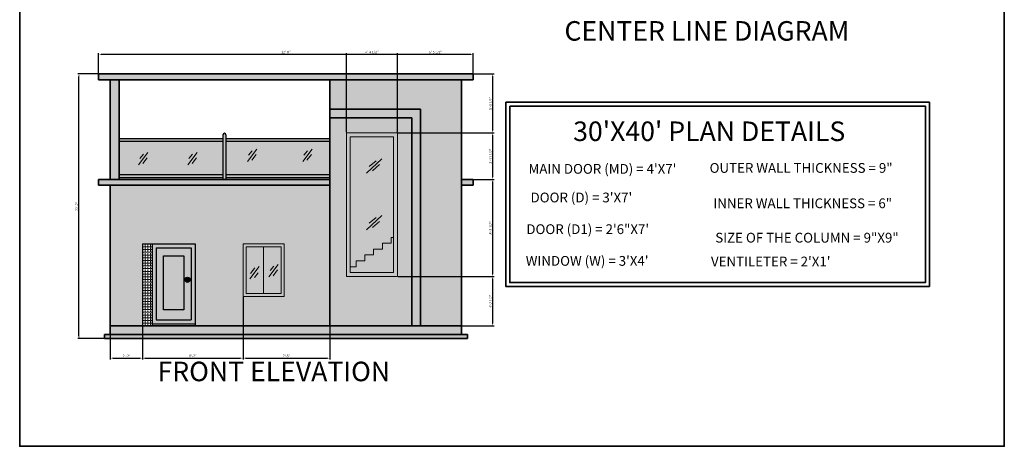
# Model space of a CAD drawing. Units: inches. Extents: x 2150 to 10686, y 1035 to 5077.
# Tile 1 of 12: x 2150 to 3159, y 1035 to 1472. Entities that reach past the tile are written whole.
import ezdxf

# ---------------------------------------------------------------- set-up
doc = ezdxf.new("R2010")
doc.units = ezdxf.units.IN
for name, color, linetype, lineweight in [('A-ANNO-DIMS', 2, 'Continuous', 18), ('A-ANNO-TEXT', 2, 'Continuous', 18), ('A-ANNO-TITL', 3, 'Continuous', 35), ('A-ANNO-TTLB', 7, 'Continuous', 35), ('A-ELEV', 7, 'Continuous', 35), ('A-ELEV-BASE-PATT', 251, 'Continuous', 13), ('A-ELEV-DOOR', 7, 'Continuous', 25), ('A-ELEV-DOOR-PATT', 17, 'Continuous', 13), ('A-ELEV-GLAZ', 7, 'Continuous', 18), ('A-ELEV-MASN-PATT', 32, 'Continuous', 13), ('A-ELEV-METL-PATT', 252, 'Continuous', 13), ('A-ELEV-RAIL', 7, 'Continuous', 25), ('A-ELEV-STRS', 7, 'Continuous', 18)]:
    doc.layers.add(name, color=color, linetype=linetype, lineweight=lineweight)
for name, color, linetype, lineweight, true_color in [('A-ELEV-CONC-PATT', 253, 'Continuous', 13, 0xb2a88f), ('A-ELEV-GLAZ-PATT', 141, 'Continuous', 13, 0xadddf7), ('A-ELEV-PATT', 253, 'Continuous', 13, 0xa5adc8)]:
    doc.layers.add(name, color=color, linetype=linetype, lineweight=lineweight, true_color=true_color)
doc.styles.get("Standard").update_dxf_attribs({"font": 'arial.ttf'})
doc.dimstyles.new('ISO-25', dxfattribs={"dimtxt": 2.5, "dimasz": 2.5, "dimexe": 1.25, "dimexo": 0.625, "dimtad": 1, "dimdec": 0, "dimlunit": 3, "dimtxsty": 'Standard', "dimcen": 2.5, "dimadec": 0, "dimazin": 0, "dimtfac": 1, "dimtdec": 0, "dimtmove": 0, "dimatfit": 3, "dimfxl": 1, "dimarcsym": 0})
pattern_1 = [(50, (-2138.8083, -54.4876), (3.6436934, -0.3187817), [0.381, -4.191]), (355, (-2138.8083, -54.4876), (-0.7048684, 3.821137), [0.3048, -3.3528117]), (100.451445, (-2138.5047, -54.514), (2.938825, 3.502355), [0.3238002, -3.561805]), (46.1842, (-2138.8083, -53.4716), (5.421581, -0.8408466), [0.5715, -6.2865]), (96.63556, (-2138.3565, -53.5416), (4.7480827, 4.9485225), [0.4857005, -5.342712]), (351.18415, (-2138.8083, -53.4716), (4.7480827, 4.9485225), [0.4571993, -5.0291946]), (21, (-2138.3003, -53.7256), (3.0322878, -2.045304), [0.381, -4.191]), (326, (-2138.3003, -53.7256), (1.2360406, 3.6837593), [0.3048, -3.3528]), (71.451445, (-2138.0476, -53.896), (4.2683284, 1.6384554), [0.3238002, -3.5617988]), (37.5, (-2138.8083, -54.4876), (0.06177207, 1.69110078), [0, -3.31216, 0, -3.4036, 0, -3.3655]), (7.5, (-2138.8083, -54.4876), (1.33639325, 2.0036115), [0, -1.94056, 0, -3.23596, 0, -1.2827]), (327.5, (-2139.9412, -54.4876), (2.7118119, -0.11457488), [0, -1.27, 0, -3.9624, 0, -5.2578]), (317.5, (-2140.4492, -54.4876), (2.9625836, 0.5085298), [0, -1.651, 0, -2.63144, 0, -3.7338])]

# ---------------------------------------------------------------- blocks, each defined once
blk = doc.blocks.new('GLASS-REFLECTION-SLIM')
for p, q in [((0, 0), (9.4, 12.8)), ((0.6, 5.5), (5.1, 11.4)), ((4.6, 1.7), (8.3, 6.2))]:
    blk.add_line(p, q)
blk = doc.blocks.new('GLASS-REFLECTION-TALL')
for p, q in [((0, 0), (15.7, 14.7)), ((2.4, 6.8), (9.9, 12.7)), ((6.1, 2.4), (13.3, 8.7))]:
    blk.add_line(p, q)
blk = doc.blocks.new('*D103')
at = {"layer": 'A-ANNO-DIMS', "color": 0, "lineweight": -2, "transparency": 16777216}
for p, q in [((2230.7, 1416.8), (2230.7, 1437.5)), ((2233.2, 1436.3), (2612.2, 1436.3)), ((2614.7, 1416.8), (2614.7, 1437.5))]:
    blk.add_line(p, q, dxfattribs=at)
at = {"layer": 'A-ANNO-DIMS', "color": 0, "transparency": 16777216}
for points in [[(2233.2, 1436.7), (2233.2, 1435.9), (2230.7, 1436.3)], [(2612.2, 1436.7), (2612.2, 1435.9), (2614.7, 1436.3)]]:
    blk.add_solid(points, dxfattribs=at)
at = {"layer": 'Defpoints', "color": 0, "transparency": 16777216}
for p in [(2614.7, 1436.3), (2230.7, 1416.2), (2614.7, 1416.2)]:
    blk.add_point(p, dxfattribs=at)
at = {"layer": 'A-ANNO-DIMS', "color": 0, "transparency": 16777216, "insert": (2422.7, 1438.2), "char_height": 2.5, "attachment_point": 5}
blk.add_mtext('32\'-0"', dxfattribs=at)
blk = doc.blocks.new('*D104')
at = {"layer": 'A-ANNO-DIMS', "color": 0, "lineweight": -2, "transparency": 16777216}
for p, q in [((2230.1, 1416.2), (2209.4, 1416.2)), ((2210.6, 1147.7), (2210.6, 1413.7)), ((2236.1, 1145.2), (2209.4, 1145.2))]:
    blk.add_line(p, q, dxfattribs=at)
at = {"layer": 'A-ANNO-DIMS', "color": 0, "transparency": 16777216}
for points in [[(2210.2, 1413.7), (2211.1, 1413.7), (2210.6, 1416.2)], [(2210.2, 1147.7), (2211.1, 1147.7), (2210.6, 1145.2)]]:
    blk.add_solid(points, dxfattribs=at)
at = {"layer": 'Defpoints', "color": 0, "transparency": 16777216}
for p in [(2210.6, 1416.2), (2230.7, 1416.2), (2236.7, 1145.2)]:
    blk.add_point(p, dxfattribs=at)
at = {"layer": 'A-ANNO-DIMS', "color": 0, "transparency": 16777216, "insert": (2208.8, 1280.7), "char_height": 2.5, "attachment_point": 5, "rotation": 90}
blk.add_mtext('22\'-7"', dxfattribs=at)
blk = doc.blocks.new('*D105')
at = {"layer": 'A-ANNO-DIMS', "color": 0, "lineweight": -2, "transparency": 16777216}
for p, q in [((2537.6, 1208.8), (2636, 1208.8)), ((2634.7, 1160.7), (2634.7, 1206.3)), ((2603.3, 1158.2), (2636, 1158.2))]:
    blk.add_line(p, q, dxfattribs=at)
at = {"layer": 'A-ANNO-DIMS', "color": 0, "transparency": 16777216}
for points in [[(2634.3, 1206.3), (2635.2, 1206.3), (2634.7, 1208.8)], [(2634.3, 1160.7), (2635.2, 1160.7), (2634.7, 1158.2)]]:
    blk.add_solid(points, dxfattribs=at)
at = {"layer": 'Defpoints', "color": 0, "transparency": 16777216}
for p in [(2537, 1208.8), (2634.7, 1208.8), (2602.7, 1158.2)]:
    blk.add_point(p, dxfattribs=at)
at = {"layer": 'A-ANNO-DIMS', "color": 0, "transparency": 16777216, "insert": (2632.8, 1183.5), "char_height": 2.5, "attachment_point": 5, "rotation": 90}
blk.add_mtext('4\'-2 1/2"', dxfattribs=at)
blk = doc.blocks.new('*D106')
at = {"layer": 'A-ANNO-DIMS', "color": 0, "lineweight": -2, "transparency": 16777216}
for p, q in [((2615.3, 1308.2), (2636, 1308.2)), ((2634.7, 1211.3), (2634.7, 1305.7)), ((2537.6, 1208.8), (2636, 1208.8))]:
    blk.add_line(p, q, dxfattribs=at)
at = {"layer": 'A-ANNO-DIMS', "color": 0, "transparency": 16777216}
for points in [[(2634.3, 1305.7), (2635.2, 1305.7), (2634.7, 1308.2)], [(2634.3, 1211.3), (2635.2, 1211.3), (2634.7, 1208.8)]]:
    blk.add_solid(points, dxfattribs=at)
at = {"layer": 'Defpoints', "color": 0, "transparency": 16777216}
for p in [(2614.7, 1308.2), (2634.7, 1308.2), (2537, 1208.8)]:
    blk.add_point(p, dxfattribs=at)
at = {"layer": 'A-ANNO-DIMS', "color": 0, "transparency": 16777216, "insert": (2632.8, 1258.5), "char_height": 2.5, "attachment_point": 5, "rotation": 90}
blk.add_mtext('8\'-3 1/2"', dxfattribs=at)
blk = doc.blocks.new('*D107')
at = {"layer": 'A-ANNO-DIMS', "color": 0, "lineweight": -2, "transparency": 16777216}
for p, q in [((2537.6, 1355.9), (2636, 1355.9)), ((2634.7, 1310.7), (2634.7, 1353.4)), ((2615.3, 1308.2), (2636, 1308.2))]:
    blk.add_line(p, q, dxfattribs=at)
at = {"layer": 'A-ANNO-DIMS', "color": 0, "transparency": 16777216}
for points in [[(2634.3, 1353.4), (2635.2, 1353.4), (2634.7, 1355.9)], [(2634.3, 1310.7), (2635.2, 1310.7), (2634.7, 1308.2)]]:
    blk.add_solid(points, dxfattribs=at)
at = {"layer": 'Defpoints', "color": 0, "transparency": 16777216}
for p in [(2537, 1355.9), (2634.7, 1355.9), (2614.7, 1308.2)]:
    blk.add_point(p, dxfattribs=at)
at = {"layer": 'A-ANNO-DIMS', "color": 0, "transparency": 16777216, "insert": (2632.8, 1332), "char_height": 2.5, "attachment_point": 5, "rotation": 90}
blk.add_mtext('3\'-11 1/2"', dxfattribs=at)
blk = doc.blocks.new('*D108')
at = {"layer": 'A-ANNO-DIMS', "color": 0, "lineweight": -2, "transparency": 16777216}
for p, q in [((2615.3, 1416.2), (2636, 1416.2)), ((2634.7, 1358.4), (2634.7, 1413.7)), ((2537.6, 1355.9), (2636, 1355.9))]:
    blk.add_line(p, q, dxfattribs=at)
at = {"layer": 'A-ANNO-DIMS', "color": 0, "transparency": 16777216}
for points in [[(2634.3, 1413.7), (2635.2, 1413.7), (2634.7, 1416.2)], [(2634.3, 1358.4), (2635.2, 1358.4), (2634.7, 1355.9)]]:
    blk.add_solid(points, dxfattribs=at)
at = {"layer": 'Defpoints', "color": 0, "transparency": 16777216}
for p in [(2614.7, 1416.2), (2634.7, 1416.2), (2537, 1355.9)]:
    blk.add_point(p, dxfattribs=at)
at = {"layer": 'A-ANNO-DIMS', "color": 0, "transparency": 16777216, "insert": (2632.8, 1386), "char_height": 2.5, "attachment_point": 5, "rotation": 90}
blk.add_mtext('5\'-0 1/2"', dxfattribs=at)
blk = doc.blocks.new('*D109')
at = {"layer": 'A-ANNO-DIMS', "color": 0, "lineweight": -2, "transparency": 16777216}
for p, q in [((2484.7, 1356.5), (2484.7, 1437.5)), ((2487.2, 1436.3), (2534.5, 1436.3)), ((2537, 1356.5), (2537, 1437.5))]:
    blk.add_line(p, q, dxfattribs=at)
at = {"layer": 'A-ANNO-DIMS', "color": 0, "transparency": 16777216}
for points in [[(2487.2, 1436.7), (2487.2, 1435.9), (2484.7, 1436.3)], [(2534.5, 1436.7), (2534.5, 1435.9), (2537, 1436.3)]]:
    blk.add_solid(points, dxfattribs=at)
at = {"layer": 'Defpoints', "color": 0, "transparency": 16777216}
for p in [(2537, 1436.3), (2484.7, 1355.9), (2537, 1355.9)]:
    blk.add_point(p, dxfattribs=at)
at = {"layer": 'A-ANNO-DIMS', "color": 0, "transparency": 16777216, "insert": (2510.9, 1438.2), "char_height": 2.5, "attachment_point": 5}
blk.add_mtext('4\'-4 1/2"', dxfattribs=at)
blk = doc.blocks.new('*D110')
at = {"layer": 'A-ANNO-DIMS', "color": 0, "lineweight": -2, "transparency": 16777216}
for p, q in [((2537, 1356.5), (2537, 1437.5)), ((2539.5, 1436.3), (2612.2, 1436.3)), ((2614.7, 1416.8), (2614.7, 1437.5))]:
    blk.add_line(p, q, dxfattribs=at)
at = {"layer": 'A-ANNO-DIMS', "color": 0, "transparency": 16777216}
for points in [[(2539.5, 1436.7), (2539.5, 1435.9), (2537, 1436.3)], [(2612.2, 1436.7), (2612.2, 1435.9), (2614.7, 1436.3)]]:
    blk.add_solid(points, dxfattribs=at)
at = {"layer": 'Defpoints', "color": 0, "transparency": 16777216}
for p in [(2614.7, 1436.3), (2614.7, 1416.2), (2537, 1355.9)]:
    blk.add_point(p, dxfattribs=at)
at = {"layer": 'A-ANNO-DIMS', "color": 0, "transparency": 16777216, "insert": (2575.9, 1438.2), "char_height": 2.5, "attachment_point": 5}
blk.add_mtext('6\'-5 1/2"', dxfattribs=at)
blk = doc.blocks.new('*D111')
at = {"layer": 'A-ANNO-DIMS', "color": 0, "lineweight": -2, "transparency": 16777216}
for p, q in [((2242.7, 1157.6), (2242.7, 1123.9)), ((2275.7, 1157.6), (2275.7, 1123.9)), ((2245.2, 1125.2), (2273.2, 1125.2))]:
    blk.add_line(p, q, dxfattribs=at)
at = {"layer": 'A-ANNO-DIMS', "color": 0, "transparency": 16777216}
for points in [[(2245.2, 1125.6), (2245.2, 1124.8), (2242.7, 1125.2)], [(2273.2, 1125.6), (2273.2, 1124.8), (2275.7, 1125.2)]]:
    blk.add_solid(points, dxfattribs=at)
at = {"layer": 'Defpoints', "color": 0, "transparency": 16777216}
for p in [(2242.7, 1158.2), (2275.7, 1158.2), (2275.7, 1125.2)]:
    blk.add_point(p, dxfattribs=at)
at = {"layer": 'A-ANNO-DIMS', "color": 0, "transparency": 16777216, "insert": (2259.2, 1127.1), "char_height": 2.5, "attachment_point": 5}
blk.add_mtext('2\'-9"', dxfattribs=at)
blk = doc.blocks.new('*D112')
at = {"layer": 'A-ANNO-DIMS', "color": 0, "lineweight": -2, "transparency": 16777216}
for p, q in [((2378.8, 1187.6), (2378.8, 1123.9)), ((2275.7, 1157.6), (2275.7, 1123.9)), ((2278.2, 1125.2), (2376.3, 1125.2))]:
    blk.add_line(p, q, dxfattribs=at)
at = {"layer": 'A-ANNO-DIMS', "color": 0, "transparency": 16777216}
for points in [[(2278.2, 1125.6), (2278.2, 1124.8), (2275.7, 1125.2)], [(2376.3, 1125.6), (2376.3, 1124.8), (2378.8, 1125.2)]]:
    blk.add_solid(points, dxfattribs=at)
at = {"layer": 'Defpoints', "color": 0, "transparency": 16777216}
for p in [(2378.8, 1188.2), (2275.7, 1158.2), (2378.8, 1125.2)]:
    blk.add_point(p, dxfattribs=at)
at = {"layer": 'A-ANNO-DIMS', "color": 0, "transparency": 16777216, "insert": (2327.3, 1127.1), "char_height": 2.5, "attachment_point": 5}
blk.add_mtext('8\'-7"', dxfattribs=at)
blk = doc.blocks.new('*D113')
at = {"layer": 'A-ANNO-DIMS', "color": 0, "lineweight": -2, "transparency": 16777216}
for p, q in [((2378.8, 1187.6), (2378.8, 1123.9)), ((2467.7, 1157.6), (2467.7, 1123.9)), ((2381.3, 1125.2), (2465.2, 1125.2))]:
    blk.add_line(p, q, dxfattribs=at)
at = {"layer": 'A-ANNO-DIMS', "color": 0, "transparency": 16777216}
for points in [[(2381.3, 1125.6), (2381.3, 1124.8), (2378.8, 1125.2)], [(2465.2, 1125.6), (2465.2, 1124.8), (2467.7, 1125.2)]]:
    blk.add_solid(points, dxfattribs=at)
at = {"layer": 'Defpoints', "color": 0, "transparency": 16777216}
for p in [(2378.8, 1188.2), (2467.7, 1158.2), (2467.7, 1125.2)]:
    blk.add_point(p, dxfattribs=at)
at = {"layer": 'A-ANNO-DIMS', "color": 0, "transparency": 16777216, "insert": (2423.3, 1127.1), "char_height": 2.5, "attachment_point": 5}
blk.add_mtext('7\'-5"', dxfattribs=at)

msp = doc.modelspace()

# ---------------------------------------------------------------- hatches: boundary and pattern name
at = {"layer": 'A-ELEV-BASE-PATT'}
h = msp.add_hatch(color=256, dxfattribs=at)
h.dxf.hatch_style = 1
h.paths.add_polyline_path([(2242.69, 1158.22), (2242.69, 1149.22), (2602.69, 1149.22), (2602.69, 1158.22)])
h = msp.add_hatch(color=256, dxfattribs=at)
h.dxf.hatch_style = 1
h.paths.add_polyline_path([(2608.69, 1145.22), (2608.69, 1149.22), (2236.69, 1149.22), (2236.69, 1145.22)])
at = {"layer": 'A-ELEV-CONC-PATT'}
h = msp.add_hatch(dxfattribs=at)
h.set_pattern_fill('AR-CONC', color=256, scale=0.02)
h.set_pattern_definition(pattern_1)
h.paths.add_polyline_path([(2230.69, 1416.22), (2230.69, 1410.22), (2614.69, 1410.22), (2614.69, 1416.22)])
h.paths.add_polyline_path([(2230.69, 1308.22), (2230.69, 1302.22), (2467.69, 1302.22), (2467.69, 1308.22)])
h.paths.add_polyline_path([(2602.69, 1308.22), (2602.69, 1302.22), (2614.69, 1302.22), (2614.69, 1308.22)])
h = msp.add_hatch(dxfattribs=at)
h.set_pattern_fill('AR-CONC', color=256, scale=0.02)
h.set_pattern_definition(pattern_1)
h.paths.add_polyline_path([(2551.69, 1158.22), (2560.69, 1158.22), (2560.69, 1380.22), (2467.69, 1380.22), (2467.69, 1371.22), (2551.69, 1371.22)])
at = {"layer": 'A-ELEV-DOOR-PATT'}
h = msp.add_hatch(color=256, dxfattribs=at)
h.dxf.hatch_style = 1
h.paths.add_polyline_path([(2329.69, 1242.22), (2285.69, 1242.22), (2285.69, 1160.22), (2329.69, 1160.22)])
h.paths.add_polyline_path([(2325.69, 1238.22), (2325.69, 1164.22), (2289.69, 1164.22), (2289.69, 1238.22)], flags=16)
h.paths.add_polyline_path([(2297.37, 1229.76), (2318.24, 1229.76), (2318.24, 1174.48), (2297.37, 1174.48)], flags=0)
h.paths.add_polyline_path([(2324.57, 1205.39, -1), (2319.32, 1205.39, -1)], flags=0)
h.paths.add_polyline_path([(2323.57, 1205.39, -1), (2320.32, 1205.39, -1)], flags=0)
h.paths.add_polyline_path([(2318.24, 1229.76), (2297.37, 1229.76), (2297.37, 1174.48), (2318.24, 1174.48)], flags=0)
h = msp.add_hatch(color=256, dxfattribs=at)
h.dxf.hatch_style = 1
h.paths.add_polyline_path([(2289.69, 1238.22), (2289.69, 1164.22), (2325.69, 1164.22), (2325.69, 1238.22)])
h.paths.add_polyline_path([(2318.24, 1229.76), (2318.24, 1174.48), (2297.37, 1174.48), (2297.37, 1229.76)], flags=16)
h.paths.add_polyline_path([(2324.57, 1205.39, -1), (2319.32, 1205.39, -1)], flags=16)
h.paths.add_polyline_path([(2323.57, 1205.39, -1), (2320.32, 1205.39, -1)], flags=0)
h = msp.add_hatch(color=256, dxfattribs=at)
h.dxf.hatch_style = 1
h.paths.add_polyline_path([(2318.24, 1229.76), (2297.37, 1229.76), (2297.37, 1174.48), (2318.24, 1174.48)])
at = {"layer": 'A-ELEV-GLAZ-PATT'}
h = msp.add_hatch(color=256, dxfattribs=at)
h.dxf.hatch_style = 1
h.paths.add_polyline_path([(2361.19, 1347.22), (2361.19, 1313.22), (2467.69, 1313.22), (2467.69, 1347.22)])
h.paths.add_polyline_path([(2358.19, 1313.22), (2358.19, 1347.22), (2251.69, 1347.22), (2251.69, 1313.22)])
h = msp.add_hatch(color=256, dxfattribs=at)
h.dxf.hatch_style = 1
h.paths.add_polyline_path([(2533.01, 1351.87), (2488.74, 1351.87), (2488.74, 1218.77), (2494.65, 1218.77), (2494.65, 1224.77), (2503.65, 1224.77), (2503.65, 1230.77), (2512.65, 1230.77), (2512.65, 1236.77), (2521.65, 1236.77), (2521.65, 1242.77), (2530.65, 1242.77), (2530.65, 1248.77), (2533.01, 1248.77)])
h.paths.add_polyline_path([(2533.01, 1248.77), (2530.65, 1248.77), (2530.65, 1242.77), (2521.65, 1242.77), (2521.65, 1236.77), (2512.65, 1236.77), (2512.65, 1230.77), (2503.65, 1230.77), (2503.65, 1224.77), (2494.65, 1224.77), (2494.65, 1218.77), (2488.74, 1218.77), (2488.74, 1212.77), (2533.01, 1212.77)])
h = msp.add_hatch(color=256, dxfattribs=at)
h.dxf.hatch_style = 1
h.paths.add_polyline_path([(2399.82, 1239.22), (2381.82, 1239.22), (2381.82, 1191.22), (2399.82, 1191.22)])
h.paths.add_polyline_path([(2417.82, 1239.22), (2399.82, 1239.22), (2399.82, 1191.22), (2417.82, 1191.22)])
at = {"layer": 'A-ELEV-MASN-PATT'}
h = msp.add_hatch(dxfattribs=at)
h.set_pattern_fill('GRAVEL', color=256, scale=0.4)
h.set_pattern_definition([(228.012788, (-2131.4931, -44.3276), (-81.28000001, -91.44), [1.366886, -135.321935]), (184.969741, (-2132.4075, -45.34357), (121.91999995, 10.16000058), [2.345619, -232.216196]), (132.510447, (-2134.7443, -45.5468), (101.60000004, -111.75999996), [1.653926, -163.738891]), (267.273689, (-2138.7067, -48.08677), (10.16000002, 203.2), [2.136018, -211.46575]), (292.833654, (-2138.8083, -50.22037), (-50.800000004, 121.92), [2.094535, -207.35923]), (357.273689, (-2137.9955, -52.15077), (-203.2, 10.16000002), [2.136018, -211.46575]), (37.6942405, (-2135.8619, -52.25237), (-132.079999994, -101.600000008), [2.824775, -279.652461]), (72.255328, (-2133.6267, -50.52517), (71.12000002, 223.519999994), [2.666878, -264.021026]), (121.429566, (-2132.8139, -47.98517), (-81.28000001, 132.079999993), [2.143252, -212.182183]), (175.236358, (-2133.9315, -46.1564), (111.76, -10.16000002), [2.446853, -119.895748]), (222.397438, (-2136.3699, -45.95317), (-121.919999996, -111.760000004), [3.164312, -313.26709]), (138.814075, (-2128.6483, -48.1884), (-71.12, 60.96), [1.080018, -106.922263]), (171.469234, (-2129.4611, -47.47717), (132.080000004, -20.319999977), [2.054728, -203.418556]), (225, (-2131.493, -47.1724), (-1e-15, -10.16), [1.436837, -12.931572]), (203.19859, (-2132.2043, -45.9532), (50.8, 20.32), [0.773765, -76.60249]), (291.80141, (-2132.9155, -46.258), (-10.16, 30.48), [1.094262, -53.619012]), (30.963757, (-2132.5091, -47.274), (30.48, 20.32), [1.777279, -57.465193]), (161.56505, (-2130.985, -46.3596), (20.32, -10.16), [1.285149, -30.843592]), (16.38954, (-2138.8083, -46.258), (101.6, 30.48), [1.800352, -178.235307]), (70.346176, (-2137.0811, -45.75), (-40.64, -111.76), [1.510396, -149.528863]), (293.19859, (-2130.9851, -44.3276), (-20.32, 50.8), [1.54752, -75.828734]), (343.61046, (-2130.3755, -45.75), (-101.6, 30.47999999), [1.800352, -178.235307]), (339.443955, (-2138.8083, -52.5572), (-50.8, 20.32), [1.73614, -85.070937]), (294.77514, (-2137.1827, -53.1668), (-50.80000006, 111.75999997), [1.454688, -144.014374]), (66.80141, (-2130.8835, -54.4876), (20.32, 50.8), [1.54752, -75.828734]), (17.354025, (-2130.2739, -53.0652), (-132.08, -40.64000001), [1.70313, -168.609504]), (69.443955, (-2135.8619, -54.4876), (-20.32, -50.8), [0.86807, -85.939008]), (101.309932, (-2131.4931, -54.4876), (-10.16, 40.64), [0.518058, -51.28798]), (165.963757, (-2131.5947, -53.9796), (30.48, -10.16), [2.094535, -39.796218]), (186.009006, (-2133.6267, -53.47157), (101.6, 10.160000005), [1.941068, -192.16546]), (303.69007, (-2132.509, -48.1884), (-10.16, 20.32), [1.465296, -35.167105]), (353.157227, (-2131.6963, -49.40757), (172.72, -20.31999999), [2.558227, -253.264036]), (60.945396, (-2129.1563, -49.7124), (-40.64, -71.12), [1.046033, -103.55757]), (90, (-2128.648, -48.798), (-10.16, 10.16), [0.6096, -9.5504]), (120.256437, (-2133.8299, -53.1668), (40.64, -71.12), [1.411468, -139.735763]), (48.012787, (-2134.5411, -51.9476), (81.28000001, 91.43999999), [2.733772, -133.955049]), (0, (-2132.712, -49.916), (10.16, 10.16), [2.6416, -7.5184]), (325.304846, (-2130.0707, -49.9156), (101.60000004, -71.119999945), [1.606438, -159.037267]), (254.054604, (-2128.7499, -50.83), (-10.16, -40.64), [1.479316, -72.4866]), (207.645975, (-2129.1563, -52.25237), (-193.040000007, -101.599999987), [2.40858, -238.449858]), (175.426079, (-2131.2899, -53.36997), (-132.08, 10.16), [2.548118, -252.263386])])
h.paths.add_polyline_path([(2602.69, 1410.22), (2467.69, 1410.22), (2467.69, 1380.22), (2560.69, 1380.22), (2560.69, 1158.22), (2602.69, 1158.22)])
h = msp.add_hatch(dxfattribs=at)
h.set_pattern_fill('ANGLE', color=256, scale=0.4)
h.set_pattern_definition([(0, (-2138.8083, -54.4876), (0, 2.794), [2.032, -0.762]), (90, (-2138.8083, -54.4876), (-2.794, 2e-16), [2.032, -0.762])])
h.paths.add_polyline_path([(2285.69, 1242.22), (2275.69, 1242.22), (2275.69, 1158.22), (2285.69, 1158.22)])
at = {"layer": 'A-ELEV-METL-PATT'}
h = msp.add_hatch(color=256, dxfattribs=at)
h.dxf.hatch_style = 1
h.paths.add_polyline_path([(2358.19, 1308.22), (2361.19, 1308.22), (2361.19, 1353.94, 1), (2358.19, 1353.94)])
h = msp.add_hatch(color=256, dxfattribs=at)
h.dxf.hatch_style = 1
h.paths.add_polyline_path([(2484.74, 1208.77), (2537.01, 1208.77), (2537.01, 1355.87), (2484.74, 1355.87)])
h.paths.add_polyline_path([(2488.74, 1351.87), (2533.01, 1351.87), (2533.01, 1212.77), (2488.74, 1212.77)], flags=16)
h = msp.add_hatch(color=256, dxfattribs=at)
h.dxf.hatch_style = 1
h.paths.add_polyline_path([(2358.19, 1350.22), (2251.69, 1350.22), (2251.69, 1347.22), (2358.19, 1347.22)])
h.paths.add_polyline_path([(2358.19, 1313.22), (2251.69, 1313.22), (2251.69, 1310.22), (2358.19, 1310.22)])
h.paths.add_polyline_path([(2467.69, 1350.22), (2361.19, 1350.22), (2361.19, 1347.22), (2467.69, 1347.22)])
h.paths.add_polyline_path([(2467.69, 1313.22), (2361.19, 1313.22), (2361.19, 1310.22), (2467.69, 1310.22)])
h = msp.add_hatch(color=256, dxfattribs=at)
h.dxf.hatch_style = 1
h.paths.add_polyline_path([(2378.82, 1242.22), (2378.82, 1188.22), (2420.82, 1188.22), (2420.82, 1242.22)])
h.paths.add_polyline_path([(2381.82, 1239.22), (2417.82, 1239.22), (2417.82, 1191.22), (2381.82, 1191.22)], flags=16)
h = msp.add_hatch(color=256, dxfattribs=at)
h.dxf.hatch_style = 1
h.paths.add_polyline_path([(2319.32, 1205.39, 1), (2324.57, 1205.39, 1)])
h.paths.add_polyline_path([(2323.57, 1205.39, -1), (2320.32, 1205.39, -1)], flags=0)
h.paths.add_polyline_path([(2323.57, 1205.39, 1), (2320.32, 1205.39, 1)], flags=16)
h = msp.add_hatch(color=256, dxfattribs=at)
h.dxf.hatch_style = 1
h.paths.add_polyline_path([(2323.57, 1205.39, 1), (2320.32, 1205.39, 1)])
at = {"layer": 'A-ELEV-PATT'}
h = msp.add_hatch(color=256, dxfattribs=at)
h.dxf.hatch_style = 1
h.paths.add_polyline_path([(2242.69, 1308.22), (2251.69, 1308.22), (2251.69, 1410.22), (2242.69, 1410.22)])
h = msp.add_hatch(color=256, dxfattribs=at)
h.dxf.hatch_style = 1
h.paths.add_polyline_path([(2551.69, 1158.22), (2551.69, 1371.22), (2467.69, 1371.22), (2467.69, 1158.22)])
h.paths.add_polyline_path([(2484.74, 1208.77), (2484.74, 1355.87), (2537.01, 1355.87), (2537.01, 1208.77)], flags=16)
h.paths.add_polyline_path([(2488.74, 1212.77), (2488.74, 1218.77), (2488.74, 1351.87), (2533.01, 1351.87), (2533.01, 1212.77)], flags=0)
h = msp.add_hatch(color=256, dxfattribs=at)
h.dxf.hatch_style = 1
h.paths.add_polyline_path([(2242.69, 1302.22), (2242.69, 1158.22), (2275.69, 1158.22), (2275.69, 1242.22), (2329.69, 1242.22), (2329.69, 1158.22), (2467.69, 1158.22), (2467.69, 1302.22)])
h.paths.add_polyline_path([(2378.82, 1242.22), (2420.82, 1242.22), (2420.82, 1188.22), (2378.82, 1188.22)], flags=16)
h.paths.add_polyline_path([(2381.82, 1239.22), (2417.82, 1239.22), (2417.82, 1191.22), (2381.82, 1191.22)], flags=0)

# ---------------------------------------------------------------- linework, layer by layer
at = {"layer": 'A-ANNO-TTLB'}
for points in [[(2149.86, 2100.72), (3159.01, 2100.72), (3159.01, 1034.91), (2149.86, 1034.91)], [(2648.1, 1387.18), (3082.17, 1387.18), (3082.17, 1198.58), (2648.1, 1198.58)], [(2652.1, 1383.18), (3078.17, 1383.18), (3078.17, 1202.58), (2652.1, 1202.58)]]:
    msp.add_lwpolyline(points, close=True, dxfattribs=at)
at = {"layer": 'A-ELEV'}
for p, q in [((2230.69, 1416.22), (2230.69, 1410.22)), ((2230.69, 1416.22), (2614.69, 1416.22)), ((2614.69, 1416.22), (2614.69, 1410.22)), ((2230.69, 1410.22), (2614.69, 1410.22)), ((2242.69, 1410.22), (2242.69, 1308.22)), ((2251.69, 1410.22), (2251.69, 1308.22)), ((2467.69, 1410.22), (2467.69, 1158.22)), ((2602.69, 1149.22), (2602.69, 1410.22)), ((2467.69, 1380.22), (2560.69, 1380.22)), ((2560.69, 1158.22), (2560.69, 1380.22)), ((2467.69, 1371.22), (2551.69, 1371.22)), ((2551.69, 1158.22), (2551.69, 1371.22)), ((2230.69, 1308.22), (2230.69, 1302.22)), ((2230.69, 1308.22), (2467.69, 1308.22)), ((2230.69, 1302.22), (2467.69, 1302.22)), ((2242.69, 1302.22), (2242.69, 1149.22)), ((2602.69, 1308.22), (2614.69, 1308.22)), ((2602.69, 1302.22), (2614.69, 1302.22)), ((2614.69, 1308.22), (2614.69, 1302.22)), ((2242.69, 1158.22), (2602.69, 1158.22)), ((2236.69, 1149.22), (2236.69, 1145.22)), ((2236.69, 1149.22), (2608.69, 1149.22)), ((2236.69, 1145.22), (2608.69, 1145.22)), ((2608.69, 1145.22), (2608.69, 1149.22))]:
    msp.add_line(p, q, dxfattribs=at)
at = {"layer": 'A-ELEV-DOOR'}
for p, q in [((2275.69, 1242.22), (2275.69, 1158.22)), ((2275.69, 1242.22), (2329.69, 1242.22)), ((2285.69, 1242.22), (2285.69, 1158.22)), ((2329.69, 1242.22), (2329.69, 1158.22)), ((2289.69, 1238.22), (2289.69, 1164.22)), ((2289.69, 1238.22), (2325.69, 1238.22)), ((2325.69, 1238.22), (2325.69, 1164.22)), ((2289.69, 1164.22), (2325.69, 1164.22)), ((2285.69, 1160.22), (2329.69, 1160.22))]:
    msp.add_line(p, q, dxfattribs=at)
msp.add_lwpolyline([(2297.37, 1229.76), (2318.24, 1229.76), (2318.24, 1174.48), (2297.37, 1174.48)], close=True, dxfattribs=at)
for radius in [2.62, 1.62]:
    msp.add_circle((2321.95, 1205.39), radius, dxfattribs=at)
at = {"layer": 'A-ELEV-GLAZ'}
for p, q in [((2378.82, 1242.22), (2378.82, 1188.22)), ((2378.82, 1242.22), (2420.82, 1242.22)), ((2420.82, 1242.22), (2420.82, 1188.22)), ((2381.82, 1239.22), (2381.82, 1191.22)), ((2381.82, 1239.22), (2417.82, 1239.22)), ((2399.82, 1239.22), (2399.82, 1191.22)), ((2417.82, 1239.22), (2417.82, 1191.22)), ((2381.82, 1191.22), (2417.82, 1191.22)), ((2378.82, 1188.22), (2420.82, 1188.22))]:
    msp.add_line(p, q, dxfattribs=at)
for points in [[(2484.74, 1355.87), (2537.01, 1355.87), (2537.01, 1208.77), (2484.74, 1208.77)], [(2488.74, 1351.87), (2533.01, 1351.87), (2533.01, 1212.77), (2488.74, 1212.77)]]:
    msp.add_lwpolyline(points, close=True, dxfattribs=at)
at = {"layer": 'A-ELEV-RAIL'}
for p, q in [((2358.19, 1353.94), (2358.19, 1308.22)), ((2361.19, 1353.94), (2361.19, 1308.22)), ((2251.69, 1350.22), (2358.19, 1350.22)), ((2251.69, 1347.22), (2358.19, 1347.22)), ((2361.19, 1350.22), (2467.69, 1350.22)), ((2361.19, 1347.22), (2467.69, 1347.22)), ((2251.69, 1313.22), (2358.19, 1313.22)), ((2361.19, 1313.22), (2467.69, 1313.22)), ((2251.69, 1310.22), (2358.19, 1310.22)), ((2361.19, 1310.22), (2467.69, 1310.22))]:
    msp.add_line(p, q, dxfattribs=at)
msp.add_arc((2359.69, 1353.94), 1.5, 0, 180, dxfattribs=at)
at = {"layer": 'A-ELEV-STRS'}
for p, q in [((2521.65, 1242.77), (2521.65, 1236.77)), ((2521.65, 1236.77), (2521.65, 1242.77)), ((2521.65, 1242.77), (2530.65, 1242.77)), ((2530.65, 1248.77), (2530.65, 1242.77)), ((2530.65, 1242.77), (2530.65, 1248.77)), ((2530.65, 1248.77), (2533.01, 1248.77)), ((2512.65, 1236.77), (2512.65, 1230.77)), ((2512.65, 1230.77), (2512.65, 1236.77)), ((2512.65, 1236.77), (2521.65, 1236.77)), ((2494.65, 1224.77), (2494.65, 1218.77)), ((2494.65, 1218.77), (2494.65, 1224.77)), ((2494.65, 1224.77), (2503.65, 1224.77)), ((2503.65, 1230.77), (2503.65, 1224.77)), ((2503.65, 1224.77), (2503.65, 1230.77)), ((2503.65, 1230.77), (2512.65, 1230.77)), ((2488.74, 1212.77), (2488.74, 1218.77)), ((2488.74, 1218.77), (2494.65, 1218.77))]:
    msp.add_line(p, q, dxfattribs=at)

# ---------------------------------------------------------------- block references
at = {"layer": 'A-ELEV-GLAZ'}
for p, rotation in [((2281.23, 1335.67), 179.1952593557704), ((2331.76, 1335.67), 179.1952593557736), ((2392.88, 1339.22), 179.1952593557704), ((2449.52, 1339.22), 179.1952593557704), ((2414.87, 1220.93), 179.1952593557686)]:
    msp.add_blockref('GLASS-REFLECTION-SLIM', p, dxfattribs=dict(at, rotation=rotation))
for name, p in [('GLASS-REFLECTION-TALL', (2505.48, 1314.59)), ('GLASS-REFLECTION-TALL', (2505.48, 1256.48)), ('GLASS-REFLECTION-SLIM', (2385.87, 1206.2))]:
    msp.add_blockref(name, p, dxfattribs=at)

# ---------------------------------------------------------------- texts
at = {"layer": 'A-ANNO-TEXT', "char_height": 10, "attachment_point": 1}
for s, width, insert in [("MAIN DOOR (MD) = 4'X7'", 1046.29, (2671.35, 1323.95)), ('OUTER WALL THICKNESS = 9"', 376.8496, (2856.98, 1324.91)), ("DOOR (D) = 3'X7'", 304.0135, (2673.46, 1294.66)), ('INNER WALL THICKNESS = 6"', 229.9749, (2860.84, 1288.72)), ('DOOR (D1) = 2\'6"X7\'', 293.9753, (2669.15, 1262.2)), ('SIZE OF THE COLUMN = 9"X9"', 272.4913, (2862.78, 1253.49)), ("WINDOW (W) = 3'X4'", 195.37, (2668.55, 1229.75)), ("VENTILETER = 2'X1'", 234.9271, (2858.38, 1229.09))]:
    msp.add_mtext_dynamic_manual_height_columns(s, width=width, gutter_width=12.5, heights=[0], dxfattribs=dict(at, insert=insert))
at = {"layer": 'A-ANNO-TITL', "char_height": 20, "attachment_point": 1}
for s, width, insert in [('CENTER LINE DIAGRAM', 668.9491, (2708.2, 1470.23)), ("30'X40' PLAN DETAILS", 660.3294, (2717.14, 1367.47)), ('FRONT ELEVATION', 668.9491, (2291.17, 1121.53))]:
    msp.add_mtext_dynamic_manual_height_columns(s, width=width, gutter_width=12.5, heights=[0], dxfattribs=dict(at, insert=insert))

# ---------------------------------------------------------------- dimensions: what is measured, and where the dimension line sits
at = {"layer": 'A-ANNO-DIMS'}
for base, p1, p2, picture, middle in [((2614.69, 1436.27), (2230.69, 1416.22), (2614.69, 1416.22), '*D103', (2422.69, 1438.17)), ((2537.01, 1436.27), (2484.74, 1355.87), (2537.01, 1355.87), '*D109', (2510.87, 1438.19)), ((2614.69, 1436.27), (2537.01, 1355.87), (2614.69, 1416.22), '*D110', (2575.85, 1438.19)), ((2378.82, 1125.17), (2275.69, 1158.22), (2378.82, 1188.22), '*D112', (2327.26, 1127.07)), ((2467.69, 1125.17), (2378.82, 1188.22), (2467.69, 1158.22), '*D113', (2423.26, 1127.07)), ((2275.69, 1125.17), (2242.69, 1158.22), (2275.69, 1158.22), '*D111', (2259.19, 1127.07))]:
    dim = msp.add_linear_dim(base=base, p1=p1, p2=p2, dimstyle='ISO-25', override={"dimdec": 1, "dimlfac": 1, "dimrnd": 0, "dimzin": 1, "dimdsep": 46, "dimlunit": 4, "dimfrac": 2}, dxfattribs=at)
    dim.commit()
    dim.dimension.update_dxf_attribs({"geometry": picture, "text_midpoint": middle})
for base, p1, p2, picture, middle in [((2210.64, 1416.22), (2236.69, 1145.22), (2230.69, 1416.22), '*D104', (2208.76, 1280.72)), ((2634.7441, 1416.2199), (2537.0142, 1355.8701), (2614.6941, 1416.2199), '*D108', (2632.8264, 1386.045)), ((2634.7441, 1355.8701), (2614.6941, 1308.2199), (2537.0142, 1355.8701), '*D107', (2632.8256, 1332.045)), ((2634.7441, 1308.2199), (2537.0142, 1208.7688), (2614.6941, 1308.2199), '*D106', (2632.8256, 1258.4943)), ((2634.7441, 1208.7688), (2602.6941, 1158.2199), (2537.0142, 1208.7688), '*D105', (2632.8264, 1183.4943))]:
    dim = msp.add_linear_dim(base=base, p1=p1, p2=p2, angle=90, dimstyle='ISO-25', override={"dimdec": 1, "dimlfac": 1, "dimrnd": 0, "dimzin": 1, "dimdsep": 46, "dimlunit": 4, "dimfrac": 2}, dxfattribs=at)
    dim.commit()
    dim.dimension.update_dxf_attribs({"geometry": picture, "text_midpoint": middle})

doc.saveas('drawing.dxf')
